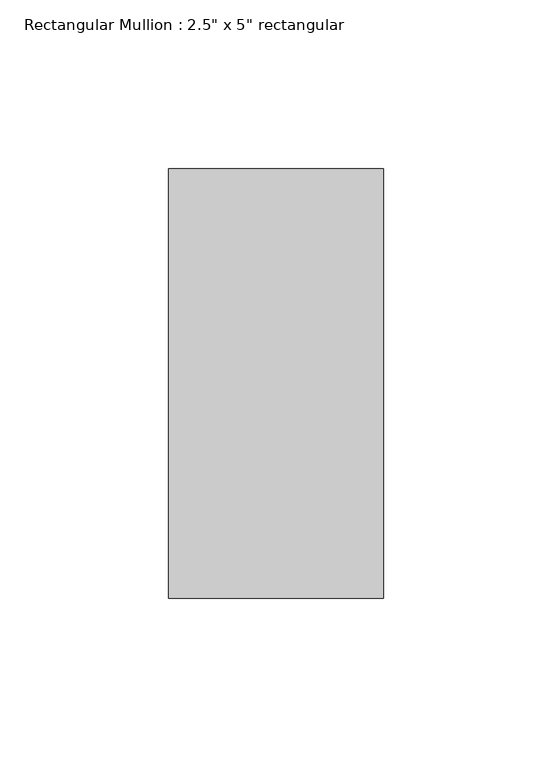
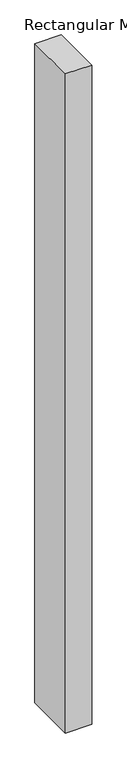
"""IFC4 building model written with IfcOpenShell, lengths in millimetres: member geometry."""

from ifc_helpers import new_model, si_unit, frame, origin, place, context, project, spatial, polyline, outline, extrude, source, transform, mapped, element, save


def member_6d86f51b(model_context):
    return source(origin(), model_context, "Body", "SweptSolid", [
        extrude(outline(polyline([(0.0, 63.5), (0.0, -63.5), (-63.5, -63.5), (-63.5, 63.5), (0.0, 63.5)])), frame((0.0, 0.0, -1675.41517), z_axis=(0.0, 0.0, 1.0), x_axis=(1.0, 0.0, 0.0)), (0.0, 0.0, 1.0), 1675.41517),
    ])


if __name__ == "__main__":
    model = new_model("IFC4")
    model_context = context("Model", 3, world=origin())
    ifc_project = project(units=[si_unit("LENGTHUNIT", "METRE", prefix="MILLI")], contexts=[model_context])
    site = spatial("IfcSite", under=ifc_project)
    building = spatial("IfcBuilding", under=site)
    placement = place(None, origin())
    member_shape = member_6d86f51b(model_context)
    element("IfcMember", 1, ObjectType="Rectangular Mullion : 2.5\" x 5\" rectangular", at=placement, inside=building, context=model_context, shape_type="MappedRepresentation", body=[
        mapped(member_shape, transform((0.0, 0.0, 0.0), x_axis=(1.0, 0.0, 0.0), y_axis=(0.0, 1.0, 0.0), z_axis=(0.0, 0.0, 1.0))),
    ])
    save(model, "model.ifc")

# Revit data of these elements
# Type "Rectangular Mullion : 2.5\" x 5\" rectangular"
#   built-in parameter 1007304 = 0.416667 (stored number, unit not read)
#   built-in parameter 1007301 = 0.104167 (stored number, unit not read)
#   built-in parameter 1007300 = 0.104167 (stored number, unit not read)
# Element 1 (IfcMember, "Rectangular Mullion : 2.5\" x 5\" rectangular")
#   Materials on its faces: "Aluminum"
# Materials
#   "Aluminum": class "Metal", colour RGB 247 247 247, transparency 0, Description = "Aluminum 6061", Cost = 0
